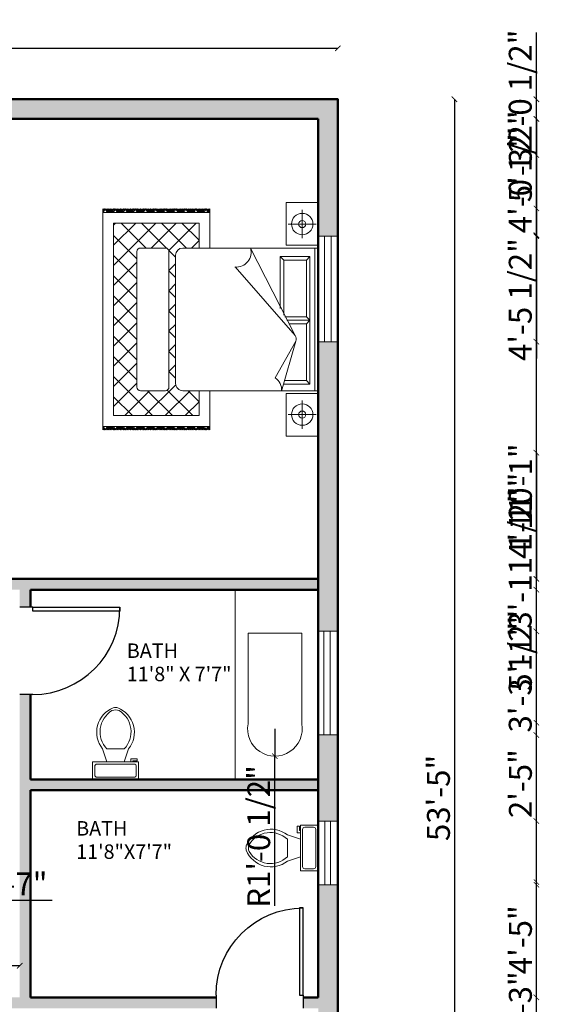
# Model space of a CAD drawing. Units: inches. Extents: x 1549 to 2410, y 1378 to 2139.
# Tile 6 of 6: x 2164 to 2410, y 1654 to 2106. Entities that reach past the tile are written whole.
import ezdxf

# ---------------------------------------------------------------- set-up
doc = ezdxf.new("R2010")
doc.units = ezdxf.units.IN
for name, color, linetype, lineweight in [('A-ANNO-DIMS', 2, 'Continuous', 18), ('A-AREA-IDEN', 7, 'Continuous', 18), ('A-DOOR', 4, 'Continuous', 25), ('A-FLOR-FIXT', 9, 'Continuous', 18), ('A-FURN', 8, 'Continuous', 18), ('A-WALL', 7, 'Continuous', 50), ('WINDOW', 2, 'Continuous', 18)]:
    doc.layers.add(name, color=color, linetype=linetype, lineweight=lineweight)
doc.layers.add('A-WALL-PATT', color=18, linetype='Continuous', lineweight=13, true_color=0x000000)
doc.styles.get("Standard").update_dxf_attribs({"font": 'arial.ttf'})
doc.dimstyles.new('ISO-25', dxfattribs={"dimtxt": 10.5, "dimasz": 2.5, "dimexe": 1.25, "dimexo": 0.625, "dimtad": 1, "dimdec": 0, "dimlunit": 4, "dimtxsty": 'Standard', "dimblk": 'ARCHTICK', "dimcen": 2.5, "dimse1": 1, "dimse2": 1, "dimclrd": 1, "dimclrt": 3, "dimadec": 0, "dimazin": 0, "dimtfac": 1, "dimtdec": 0, "dimtmove": 0, "dimatfit": 3, "dimfxl": 1, "dimarcsym": 0})

# ---------------------------------------------------------------- blocks, each defined once
blk = doc.blocks.new('*U5')
for p, q in [((9.5, -6), (9.5, -2)), ((-10, -8.5), (-8, -8.5)), ((-10, -9.5), (-10, -8.5)), ((-8, -8.5), (-8, -8)), ((-7, -8), (-7, -9.5)), ((-4, -8), (-6, -14)), ((4, -8), (6, -14)), ((-7, -9.5), (-10, -9.5)), ((4, -14), (-4, -14))]:
    blk.add_line(p, q)
blk.add_lwpolyline([(10.5, -8), (10.5, 0), (-10.5, 0), (-10.5, -8)], close=True)
for points in [[(-9.5, -2), (-9.5, -6)], [(8.5, -1), (-8.5, -1)], [(-8.5, -7), (8.5, -7)]]:
    blk.add_lwpolyline(points)
for centre, radius, start, end in [((-8.62, -1.88), 0.884, 81.8699, 188.1301), ((8.62, -1.88), 0.884, 351.8699, 98.1301), ((-8.62, -6.12), 0.884, 171.8699, 278.1301), ((8.62, -6.12), 0.884, 261.8699, 8.1301), ((3.52, -21.58), 12.17, 141.4691, 247.9714), ((4.2, -21.82), 11.33, 136.3677, 238.9468), ((-3.52, -21.58), 12.17, 292.0284, 38.5307), ((-4.2, -21.82), 11.33, 301.053, 43.6321), ((0, -27.88), 4, 245.7318, 294.2682), ((0, -29), 4, 254.8605, 285.1395)]:
    blk.add_arc(centre, radius, start, end)
blk = doc.blocks.new('*U3')
for p, q in [((0, 0), (0, -6)), ((40, 0), (40, -6))]:
    blk.add_line(p, q)
blk.add_lwpolyline([(0, 0), (0, 40), (1.75, 40), (1.75, 0)], close=True)
blk.add_arc((0, 0), 40, 0, 90)
blk = doc.blocks.new('A$C4CB008C5')
for p, q in [((0, 3.019), (0.6, 3.019)), ((0, 2.569), (0, 3.019)), ((0.304, 2.6), (0.304, 2.992)), ((0.6, 3.019), (0.6, 2.569)), ((0.64, 1.121), (0.64, 3.021)), ((0.64, 3.021), (2.64, 3.021)), ((0.64, 2.971), (2.64, 2.971)), ((0.759, 2.905), (2.547, 2.905)), ((0.759, 2.489), (0.759, 2.905)), ((0.759, 2.905), (0.809, 2.855)), ((1.603, 2.855), (1.653, 2.905)), ((1.653, 2.905), (1.653, 2.579)), ((1.653, 2.905), (1.703, 2.855)), ((2.497, 2.855), (2.547, 2.905)), ((2.547, 2.905), (2.547, 2.54)), ((2.64, 3.021), (2.64, 1.121)), ((3.279, 3.019), (2.679, 3.019)), ((2.679, 3.019), (2.679, 2.569)), ((2.975, 2.6), (2.975, 2.992)), ((3.279, 2.569), (3.279, 3.019)), ((0.106, 2.796), (0.503, 2.796)), ((0.809, 2.855), (1.603, 2.855)), ((0.809, 2.539), (0.809, 2.855)), ((1.603, 2.855), (1.603, 2.551)), ((1.703, 2.855), (1.703, 2.607)), ((1.703, 2.855), (2.497, 2.855)), ((2.497, 2.855), (2.497, 2.556)), ((3.174, 2.796), (2.776, 2.796)), ((0.64, 2.071), (1.866, 2.698)), ((0.906, 1.854), (1.866, 2.698)), ((1.946, 2.705), (2.646, 2.507)), ((1.946, 2.705), (2.46, 2.418)), ((0.6, 2.569), (0, 2.569)), ((0.809, 2.539), (0.759, 2.489)), ((1.49, 2.489), (0.759, 2.489)), ((1.58, 2.539), (0.809, 2.539)), ((2.679, 2.569), (3.279, 2.569)), ((0.907, 1.867), (0.919, 1.867)), ((0.09, 1.5), (0.64, 1.5)), ((0.09, 1.491), (0.099, 1.5)), ((0.09, 1.473), (0.116, 1.5)), ((0.09, 1.456), (0.134, 1.5)), ((0.09, 1.474), (0.09, 1.475)), ((0.09, 1.438), (0.126, 1.474)), ((0.117, 1.43), (0.09, 1.457)), ((0.14, 1.389), (0.09, 1.439)), ((0.09, 1.42), (0.099, 1.43)), ((0.14, 1.372), (0.09, 1.422)), ((0.09, 1.368), (0.14, 1.417)), ((0.14, 1.354), (0.09, 1.404)), ((0.09, 1.35), (0.14, 1.4)), ((0.14, 1.336), (0.09, 1.386)), ((0.09, 1.332), (0.14, 1.382)), ((0.14, 1.46), (0.108, 1.492)), ((0.117, 1.412), (0.14, 1.435)), ((0.14, 1.478), (0.118, 1.5)), ((0.14, 1.496), (0.135, 1.5)), ((0.14, 1.442), (0.135, 1.448)), ((0.14, 0), (0.14, 1.5)), ((2.64, 1.5), (3.19, 1.5)), ((3.14, 1.496), (3.144, 1.5)), ((3.14, 1.478), (3.162, 1.5)), ((3.14, 1.5), (3.14, 0)), ((3.14, 1.46), (3.171, 1.492)), ((3.14, 1.442), (3.145, 1.448)), ((3.14, 1.389), (3.19, 1.439)), ((3.162, 1.412), (3.14, 1.435)), ((3.14, 1.372), (3.19, 1.422)), ((3.189, 1.368), (3.14, 1.417)), ((3.14, 1.354), (3.19, 1.404)), ((3.19, 1.35), (3.14, 1.4)), ((3.14, 1.336), (3.19, 1.386)), ((3.19, 1.332), (3.14, 1.382)), ((3.19, 1.456), (3.145, 1.5)), ((3.19, 1.438), (3.154, 1.474)), ((3.162, 1.43), (3.19, 1.457)), ((3.19, 1.473), (3.163, 1.5)), ((3.19, 1.42), (3.18, 1.43)), ((3.19, 1.491), (3.181, 1.5)), ((3.189, 1.474), (3.19, 1.475)), ((0.09, 1.314), (0.14, 1.364)), ((0.09, 1.297), (0.126, 1.333)), ((0.09, 1.333), (0.09, 1.333)), ((0.117, 1.288), (0.09, 1.316)), ((0.14, 1.248), (0.09, 1.298)), ((0.09, 1.279), (0.099, 1.288)), ((0.14, 1.23), (0.09, 1.28)), ((0.09, 1.227), (0.14, 1.276)), ((0.14, 1.213), (0.09, 1.263)), ((0.09, 1.208), (0.14, 1.258)), ((0.14, 1.195), (0.09, 1.245)), ((0.14, 1.319), (0.108, 1.35)), ((0.117, 1.271), (0.14, 1.294)), ((0.14, 1.301), (0.135, 1.306)), ((0.29, 1.108), (0.532, 1.35)), ((0.29, 0.15), (0.29, 1.35)), ((0.29, 1.35), (0.64, 1.35)), ((0.674, 0.926), (0.29, 1.31)), ((0.64, 1.243), (0.533, 1.35)), ((2.632, 0.904), (2.99, 1.262)), ((2.64, 1.195), (2.795, 1.35)), ((2.64, 1.35), (2.99, 1.35)), ((2.99, 1.156), (2.795, 1.35)), ((2.99, 1.35), (2.99, 0.15)), ((3.19, 1.314), (3.14, 1.364)), ((3.14, 1.319), (3.171, 1.35)), ((3.14, 1.301), (3.145, 1.306)), ((3.14, 1.248), (3.19, 1.298)), ((3.162, 1.271), (3.14, 1.294)), ((3.14, 1.23), (3.19, 1.28)), ((3.189, 1.227), (3.14, 1.276)), ((3.14, 1.213), (3.19, 1.263)), ((3.19, 1.208), (3.14, 1.258)), ((3.14, 1.195), (3.19, 1.245)), ((3.19, 1.297), (3.154, 1.333)), ((3.162, 1.288), (3.19, 1.316)), ((3.19, 1.279), (3.18, 1.288)), ((3.189, 1.333), (3.19, 1.333)), ((0.09, 1.19), (0.14, 1.24)), ((0.09, 1.173), (0.14, 1.223)), ((0.09, 1.191), (0.09, 1.192)), ((0.09, 1.155), (0.126, 1.191)), ((0.117, 1.147), (0.09, 1.174)), ((0.14, 1.107), (0.09, 1.157)), ((0.09, 1.137), (0.099, 1.147)), ((0.14, 1.089), (0.09, 1.139)), ((0.09, 1.085), (0.14, 1.134)), ((0.14, 1.071), (0.09, 1.121)), ((0.09, 1.067), (0.14, 1.117)), ((0.14, 1.177), (0.108, 1.209)), ((0.117, 1.129), (0.14, 1.152)), ((0.14, 1.16), (0.135, 1.165)), ((0.29, 0.825), (0.64, 1.175)), ((2.99, 0.873), (2.64, 1.223)), ((3.19, 1.19), (3.14, 1.24)), ((3.19, 1.173), (3.14, 1.223)), ((3.14, 1.177), (3.171, 1.209)), ((3.14, 1.16), (3.145, 1.165)), ((3.14, 1.107), (3.19, 1.157)), ((3.162, 1.129), (3.14, 1.152)), ((3.14, 1.089), (3.19, 1.139)), ((3.189, 1.085), (3.14, 1.134)), ((3.14, 1.071), (3.19, 1.121)), ((3.19, 1.067), (3.14, 1.117)), ((3.19, 1.155), (3.154, 1.191)), ((3.162, 1.147), (3.19, 1.174)), ((3.19, 1.137), (3.18, 1.147)), ((3.189, 1.191), (3.19, 1.192)), ((0.14, 1.054), (0.09, 1.104)), ((0.09, 1.049), (0.14, 1.099)), ((0.09, 1.031), (0.14, 1.081)), ((0.09, 1.05), (0.09, 1.051)), ((0.09, 1.014), (0.126, 1.05)), ((0.117, 1.006), (0.09, 1.033)), ((0.14, 0.965), (0.09, 1.015)), ((0.09, 0.996), (0.099, 1.006)), ((0.14, 0.948), (0.09, 0.998)), ((0.09, 0.944), (0.14, 0.993)), ((0.14, 0.93), (0.09, 0.98)), ((0.09, 0.925), (0.14, 0.975)), ((0.14, 1.036), (0.108, 1.067)), ((0.117, 0.988), (0.14, 1.011)), ((0.14, 1.018), (0.135, 1.023)), ((0.64, 0.677), (0.29, 1.027)), ((0.673, 0.925), (0.769, 1.021)), ((2.54, 1.021), (0.74, 1.021)), ((0.955, 0.928), (0.861, 1.021)), ((0.959, 0.928), (1.052, 1.021)), ((1.238, 0.928), (1.144, 1.021)), ((1.241, 0.928), (1.335, 1.021)), ((1.52, 0.928), (1.427, 1.021)), ((1.524, 0.928), (1.618, 1.021)), ((1.803, 0.928), (1.71, 1.021)), ((1.807, 0.928), (1.9, 1.021)), ((2.086, 0.928), (1.993, 1.021)), ((2.09, 0.928), (2.183, 1.021)), ((2.369, 0.928), (2.276, 1.021)), ((2.373, 0.928), (2.466, 1.021)), ((2.99, 0.59), (2.557, 1.023)), ((2.64, 0.629), (2.99, 0.979)), ((3.14, 1.054), (3.19, 1.104)), ((3.19, 1.049), (3.14, 1.099)), ((3.19, 1.031), (3.14, 1.081)), ((3.14, 1.036), (3.171, 1.067)), ((3.14, 1.018), (3.145, 1.023)), ((3.14, 0.965), (3.19, 1.015)), ((3.162, 0.988), (3.14, 1.011)), ((3.14, 0.948), (3.19, 0.998)), ((3.189, 0.944), (3.14, 0.993)), ((3.14, 0.93), (3.19, 0.98)), ((3.19, 0.925), (3.14, 0.975)), ((3.19, 1.014), (3.154, 1.05)), ((3.162, 1.006), (3.19, 1.033)), ((3.19, 0.996), (3.18, 1.006)), ((3.189, 1.05), (3.19, 1.051)), ((0.14, 0.912), (0.09, 0.962)), ((0.09, 0.908), (0.14, 0.958)), ((0.09, 0.89), (0.14, 0.94)), ((0.09, 0.908), (0.09, 0.909)), ((0.09, 0.872), (0.126, 0.908)), ((0.117, 0.864), (0.09, 0.891)), ((0.14, 0.824), (0.09, 0.874)), ((0.09, 0.855), (0.099, 0.864)), ((0.14, 0.806), (0.09, 0.856)), ((0.09, 0.802), (0.14, 0.852)), ((0.14, 0.788), (0.09, 0.838)), ((0.09, 0.784), (0.14, 0.834)), ((0.14, 0.894), (0.108, 0.926)), ((0.117, 0.847), (0.14, 0.869)), ((0.14, 0.877), (0.135, 0.882)), ((0.29, 0.542), (0.643, 0.895)), ((0.64, 0.878), (0.64, 0.528)), ((0.69, 0.928), (2.59, 0.928)), ((2.64, 0.878), (2.64, 0.528)), ((3.14, 0.912), (3.19, 0.962)), ((3.19, 0.908), (3.14, 0.958)), ((3.19, 0.89), (3.14, 0.94)), ((3.14, 0.894), (3.171, 0.926)), ((3.14, 0.877), (3.145, 0.882)), ((3.14, 0.824), (3.19, 0.874)), ((3.162, 0.847), (3.14, 0.869)), ((3.14, 0.806), (3.19, 0.856)), ((3.189, 0.802), (3.14, 0.852)), ((3.14, 0.788), (3.19, 0.838)), ((3.19, 0.784), (3.14, 0.834)), ((3.19, 0.872), (3.154, 0.908)), ((3.162, 0.864), (3.19, 0.891)), ((3.19, 0.855), (3.18, 0.864)), ((3.189, 0.908), (3.19, 0.909)), ((0.14, 0.771), (0.09, 0.821)), ((0.09, 0.766), (0.14, 0.816)), ((0.09, 0.749), (0.14, 0.799)), ((0.09, 0.767), (0.09, 0.768)), ((0.09, 0.731), (0.126, 0.767)), ((0.117, 0.723), (0.09, 0.75)), ((0.14, 0.682), (0.09, 0.732)), ((0.09, 0.713), (0.099, 0.723)), ((0.14, 0.665), (0.09, 0.715)), ((0.09, 0.661), (0.14, 0.71)), ((0.14, 0.647), (0.09, 0.697)), ((0.09, 0.642), (0.14, 0.692)), ((0.14, 0.753), (0.108, 0.785)), ((0.117, 0.705), (0.14, 0.728)), ((0.14, 0.735), (0.135, 0.74)), ((0.884, 0.15), (0.29, 0.744)), ((2.443, 0.15), (2.99, 0.696)), ((3.14, 0.771), (3.19, 0.821)), ((3.19, 0.766), (3.14, 0.816)), ((3.19, 0.749), (3.14, 0.799)), ((3.14, 0.753), (3.171, 0.785)), ((3.14, 0.735), (3.145, 0.74)), ((3.14, 0.682), (3.19, 0.732)), ((3.162, 0.705), (3.14, 0.728)), ((3.14, 0.665), (3.19, 0.715)), ((3.189, 0.661), (3.14, 0.71)), ((3.14, 0.647), (3.19, 0.697)), ((3.19, 0.642), (3.14, 0.692)), ((3.19, 0.731), (3.154, 0.767)), ((3.162, 0.723), (3.19, 0.75)), ((3.19, 0.713), (3.18, 0.723)), ((3.189, 0.767), (3.19, 0.768)), ((0.14, 0.629), (0.09, 0.679)), ((0.09, 0.625), (0.14, 0.675)), ((0.09, 0.607), (0.14, 0.657)), ((0.09, 0.589), (0.126, 0.626)), ((0.09, 0.626), (0.09, 0.626)), ((0.117, 0.581), (0.09, 0.609)), ((0.14, 0.541), (0.09, 0.591)), ((0.09, 0.572), (0.099, 0.581)), ((0.14, 0.523), (0.09, 0.573)), ((0.09, 0.519), (0.14, 0.569)), ((0.14, 0.506), (0.09, 0.556)), ((0.14, 0.612), (0.108, 0.643)), ((0.117, 0.564), (0.14, 0.586)), ((0.14, 0.594), (0.135, 0.599)), ((0.29, 0.259), (0.64, 0.609)), ((2.99, 0.307), (2.64, 0.657)), ((3.14, 0.629), (3.19, 0.679)), ((3.19, 0.625), (3.14, 0.675)), ((3.19, 0.607), (3.14, 0.657)), ((3.14, 0.612), (3.171, 0.643)), ((3.14, 0.594), (3.145, 0.599)), ((3.14, 0.541), (3.19, 0.591)), ((3.162, 0.564), (3.14, 0.586)), ((3.14, 0.523), (3.19, 0.573)), ((3.189, 0.519), (3.14, 0.569)), ((3.14, 0.506), (3.19, 0.556)), ((3.19, 0.589), (3.154, 0.626)), ((3.162, 0.581), (3.19, 0.609)), ((3.19, 0.572), (3.18, 0.581)), ((3.189, 0.626), (3.19, 0.626)), ((0.09, 0.501), (0.14, 0.551)), ((0.14, 0.488), (0.09, 0.538)), ((0.09, 0.483), (0.14, 0.533)), ((0.09, 0.466), (0.14, 0.516)), ((0.09, 0.484), (0.09, 0.485)), ((0.09, 0.448), (0.126, 0.484)), ((0.117, 0.44), (0.09, 0.467)), ((0.14, 0.399), (0.09, 0.449)), ((0.09, 0.43), (0.099, 0.44)), ((0.14, 0.382), (0.09, 0.432)), ((0.09, 0.378), (0.14, 0.427)), ((0.14, 0.364), (0.09, 0.414)), ((0.14, 0.47), (0.108, 0.502)), ((0.117, 0.422), (0.14, 0.445)), ((0.14, 0.453), (0.135, 0.458)), ((0.601, 0.15), (0.29, 0.462)), ((0.463, 0.15), (0.791, 0.478)), ((0.69, 0.478), (2.59, 0.478)), ((0.746, 0.15), (1.074, 0.478)), ((1.167, 0.15), (0.839, 0.478)), ((1.029, 0.15), (1.357, 0.478)), ((1.45, 0.15), (1.122, 0.478)), ((1.312, 0.15), (1.64, 0.478)), ((1.733, 0.15), (1.405, 0.478)), ((1.595, 0.15), (1.923, 0.478)), ((2.016, 0.15), (1.688, 0.478)), ((1.878, 0.15), (2.206, 0.478)), ((2.298, 0.15), (1.97, 0.478)), ((2.16, 0.15), (2.488, 0.478)), ((2.581, 0.15), (2.253, 0.478)), ((2.864, 0.15), (2.536, 0.478)), ((3.19, 0.501), (3.14, 0.551)), ((3.14, 0.488), (3.19, 0.538)), ((3.19, 0.483), (3.14, 0.533)), ((3.19, 0.466), (3.14, 0.516)), ((3.14, 0.47), (3.171, 0.502)), ((3.14, 0.453), (3.145, 0.458)), ((3.14, 0.399), (3.19, 0.449)), ((3.162, 0.422), (3.14, 0.445)), ((3.14, 0.382), (3.19, 0.432)), ((3.189, 0.378), (3.14, 0.427)), ((3.14, 0.364), (3.19, 0.414)), ((3.19, 0.448), (3.154, 0.484)), ((3.162, 0.44), (3.19, 0.467)), ((3.19, 0.43), (3.18, 0.44)), ((3.189, 0.484), (3.19, 0.485)), ((0.09, 0.36), (0.14, 0.41)), ((0.14, 0.346), (0.09, 0.396)), ((0.09, 0.342), (0.14, 0.392)), ((0.09, 0.324), (0.14, 0.374)), ((0.09, 0.307), (0.126, 0.343)), ((0.09, 0.343), (0.09, 0.343)), ((0.117, 0.299), (0.09, 0.326)), ((0.14, 0.258), (0.09, 0.308)), ((0.09, 0.289), (0.099, 0.299)), ((0.14, 0.24), (0.09, 0.29)), ((0.09, 0.237), (0.14, 0.286)), ((0.14, 0.329), (0.108, 0.36)), ((0.117, 0.281), (0.14, 0.304)), ((0.14, 0.311), (0.135, 0.316)), ((2.726, 0.15), (2.99, 0.414)), ((3.19, 0.36), (3.14, 0.41)), ((3.14, 0.346), (3.19, 0.396)), ((3.19, 0.342), (3.14, 0.392)), ((3.19, 0.324), (3.14, 0.374)), ((3.14, 0.329), (3.171, 0.36)), ((3.14, 0.311), (3.145, 0.316)), ((3.14, 0.258), (3.19, 0.308)), ((3.162, 0.281), (3.14, 0.304)), ((3.14, 0.24), (3.19, 0.29)), ((3.189, 0.237), (3.14, 0.286)), ((3.19, 0.307), (3.154, 0.343)), ((3.162, 0.299), (3.19, 0.326)), ((3.19, 0.289), (3.18, 0.299)), ((3.189, 0.343), (3.19, 0.343)), ((0.14, 0.223), (0.09, 0.273)), ((0.09, 0.218), (0.14, 0.268)), ((0.14, 0.205), (0.09, 0.255)), ((0.09, 0.201), (0.14, 0.251)), ((0.09, 0.183), (0.14, 0.233)), ((0.09, 0.201), (0.09, 0.202)), ((0.09, 0.165), (0.126, 0.201)), ((0.117, 0.157), (0.09, 0.184)), ((0.14, 0.117), (0.09, 0.167)), ((0.09, 0.148), (0.099, 0.157)), ((0.14, 0.099), (0.09, 0.149)), ((0.09, 0.095), (0.14, 0.144)), ((0.14, 0.187), (0.108, 0.219)), ((0.117, 0.139), (0.14, 0.162)), ((0.14, 0.17), (0.135, 0.175)), ((0.318, 0.15), (0.29, 0.179)), ((2.99, 0.15), (0.29, 0.15)), ((3.14, 0.223), (3.19, 0.273)), ((3.19, 0.218), (3.14, 0.268)), ((3.14, 0.205), (3.19, 0.255)), ((3.19, 0.201), (3.14, 0.251)), ((3.19, 0.183), (3.14, 0.233)), ((3.14, 0.187), (3.171, 0.219)), ((3.14, 0.17), (3.145, 0.175)), ((3.14, 0.117), (3.19, 0.167)), ((3.162, 0.139), (3.14, 0.162)), ((3.14, 0.099), (3.19, 0.149)), ((3.189, 0.095), (3.14, 0.144)), ((3.19, 0.165), (3.154, 0.201)), ((3.162, 0.157), (3.19, 0.184)), ((3.19, 0.148), (3.18, 0.157)), ((3.189, 0.201), (3.19, 0.202)), ((0.14, 0.081), (0.09, 0.131)), ((0.09, 0.077), (0.14, 0.127)), ((0.14, 0.064), (0.09, 0.114)), ((0.09, 0.059), (0.14, 0.109)), ((0.09, 0.041), (0.14, 0.091)), ((0.09, 0.06), (0.09, 0.061)), ((0.09, 0.024), (0.126, 0.06)), ((0.117, 0.016), (0.09, 0.043)), ((0.115, 0), (0.09, 0.025)), ((0.09, 0.006), (0.099, 0.016)), ((0.097, 0), (0.09, 0.008)), ((0.14, 0.046), (0.108, 0.078)), ((0.119, 0), (0.14, 0.021)), ((0.14, 0.028), (0.135, 0.033)), ((0.137, 0), (0.14, 0.003)), ((3.14, 0.081), (3.19, 0.131)), ((3.19, 0.077), (3.14, 0.127)), ((3.14, 0.064), (3.19, 0.114)), ((3.19, 0.059), (3.14, 0.109)), ((3.19, 0.041), (3.14, 0.091)), ((3.14, 0.046), (3.171, 0.078)), ((3.14, 0.028), (3.145, 0.033)), ((3.16, 0), (3.14, 0.021)), ((3.143, 0), (3.14, 0.003)), ((3.19, 0.024), (3.154, 0.06)), ((3.162, 0.016), (3.19, 0.043)), ((3.164, 0), (3.19, 0.025)), ((3.19, 0.006), (3.18, 0.016)), ((3.182, 0), (3.19, 0.008)), ((3.189, 0.06), (3.19, 0.061)), ((0.09, 0), (3.19, 0))]:
    blk.add_line(p, q)
for centre, radius in [((0.304, 2.796), 0.15), ((2.975, 2.796), 0.15), ((0.304, 2.796), 0.05), ((2.975, 2.796), 0.05)]:
    blk.add_circle(centre, radius)
for centre, radius, start, end in [((1.915, 2.61), 0.1, 71.7215, 119.0799), ((2.626, 2.31), 0.198, 84.1725, 146.9889), ((0.7, 1.873), 0.207, 354.6422, 106.9775), ((0.74, 1.121), 0.1, 180, 270), ((2.54, 1.121), 0.1, 270, 0), ((0.69, 0.878), 0.05, 90, 180), ((2.59, 0.878), 0.05, 0, 90), ((0.69, 0.528), 0.05, 180, 270), ((2.59, 0.528), 0.05, 270, 0)]:
    blk.add_arc(centre, radius, start, end)
blk = doc.blocks.new('_ArchTick')
at = {"color": 0, "linetype": 'ByBlock', "const_width": 0.15}
blk.add_lwpolyline([(-0.5, -0.5), (0.5, 0.5)], dxfattribs=at)
blk = doc.blocks.new('*D13')
at = {"layer": 'A-ANNO-DIMS', "color": 0, "lineweight": -2, "transparency": 16777216}
blk.add_line((1688.62, 2092.38), (2309.62, 2092.38), dxfattribs=at)
at = {"layer": 'Defpoints', "color": 0, "transparency": 16777216}
for p in [(2309.62, 2092.38), (1688.62, 2069.01), (2309.62, 2069.01)]:
    blk.add_point(p, dxfattribs=at)
at = {"layer": 'A-ANNO-DIMS', "color": 0, "lineweight": -2, "transparency": 16777216, "xscale": 2.5, "yscale": 2.5, "zscale": 2.5, "rotation": 180}
blk.add_blockref('_ArchTick', (1688.62, 2092.38), dxfattribs=at)
at = {"layer": 'A-ANNO-DIMS', "color": 0, "lineweight": -2, "transparency": 16777216, "xscale": 2.5, "yscale": 2.5, "zscale": 2.5}
blk.add_blockref('_ArchTick', (2309.62, 2092.38), dxfattribs=at)
at = {"layer": 'A-ANNO-DIMS', "color": 0, "transparency": 16777216, "insert": (1999.12, 2098.36), "char_height": 10.5, "attachment_point": 5}
blk.add_mtext('51\'-9"', dxfattribs=at)
blk = doc.blocks.new('*D14')
at = {"layer": 'A-ANNO-DIMS', "color": 0, "lineweight": -2, "transparency": 16777216}
blk.add_line((2363.11, 2069.01), (2363.11, 1428.01), dxfattribs=at)
at = {"layer": 'Defpoints', "color": 0, "transparency": 16777216}
for p in [(2309.62, 2069.01), (2309.62, 1428.01), (2363.11, 1428.01)]:
    blk.add_point(p, dxfattribs=at)
at = {"layer": 'A-ANNO-DIMS', "color": 0, "lineweight": -2, "transparency": 16777216, "xscale": 2.5, "yscale": 2.5, "zscale": 2.5}
for p, rotation in [((2363.11, 2069.01), 90), ((2363.11, 1428.01), 270)]:
    blk.add_blockref('_ArchTick', p, dxfattribs=dict(at, rotation=rotation))
at = {"layer": 'A-ANNO-DIMS', "color": 0, "transparency": 16777216, "insert": (2357.12, 1748.51), "char_height": 10.5, "attachment_point": 5, "rotation": 90}
blk.add_mtext('53\'-5"', dxfattribs=at)
blk = doc.blocks.new('*D23')
at = {"layer": 'A-ANNO-DIMS', "color": 1, "lineweight": -2, "transparency": 16777216}
for p, q in [((1968.32, 1701.64), (2059.32, 1701.64)), ((2059.32, 1701.64), (2178.47, 1701.64))]:
    blk.add_line(p, q, dxfattribs=at)
at = {"layer": 'Defpoints', "color": 0, "transparency": 16777216}
for p in [(1968.32, 1715.29), (2059.32, 1715.29), (2059.32, 1701.64)]:
    blk.add_point(p, dxfattribs=at)
at = {"layer": 'A-ANNO-DIMS', "color": 1, "lineweight": -2, "transparency": 16777216, "xscale": 2.5, "yscale": 2.5, "zscale": 2.5, "rotation": 180}
blk.add_blockref('_ArchTick', (1968.32, 1701.64), dxfattribs=at)
at = {"layer": 'A-ANNO-DIMS', "color": 1, "lineweight": -2, "transparency": 16777216, "xscale": 2.5, "yscale": 2.5, "zscale": 2.5}
blk.add_blockref('_ArchTick', (2059.32, 1701.64), dxfattribs=at)
at = {"layer": 'A-ANNO-DIMS', "color": 3, "transparency": 16777216, "insert": (2120.15, 1707.7), "char_height": 10.5, "attachment_point": 5}
blk.add_mtext('DINING SET 7\'-7"', dxfattribs=at)
blk = doc.blocks.new('*D26')
at = {"layer": 'A-ANNO-DIMS', "color": 1, "lineweight": -2, "transparency": 16777216}
blk.add_line((2163.62, 1671.5), (2097.13, 1671.5), dxfattribs=at)
at = {"layer": 'Defpoints', "color": 0, "transparency": 16777216}
for p in [(2097.13, 1684.51), (2163.62, 1684.51), (2097.13, 1671.5)]:
    blk.add_point(p, dxfattribs=at)
at = {"layer": 'A-ANNO-DIMS', "color": 1, "lineweight": -2, "transparency": 16777216, "xscale": 2.5, "yscale": 2.5, "zscale": 2.5, "rotation": 180}
blk.add_blockref('_ArchTick', (2097.13, 1671.5), dxfattribs=at)
at = {"layer": 'A-ANNO-DIMS', "color": 1, "lineweight": -2, "transparency": 16777216, "xscale": 2.5, "yscale": 2.5, "zscale": 2.5}
blk.add_blockref('_ArchTick', (2163.62, 1671.5), dxfattribs=at)
at = {"layer": 'A-ANNO-DIMS', "color": 3, "transparency": 16777216, "insert": (2130.37, 1677.55), "char_height": 10.5, "attachment_point": 5}
blk.add_mtext('5\'-6 1/2"', dxfattribs=at)
blk = doc.blocks.new('*D41')
at = {"layer": 'A-ANNO-DIMS', "color": 1, "lineweight": -2, "transparency": 16777216}
blk.add_line((2400.7, 1597.64), (2400.7, 1708.66), dxfattribs=at)
at = {"layer": 'Defpoints', "color": 0, "transparency": 16777216}
for p in [(2309.62, 1708.66), (2400.7, 1708.66), (2309.62, 1597.64)]:
    blk.add_point(p, dxfattribs=at)
at = {"layer": 'A-ANNO-DIMS', "color": 1, "lineweight": -2, "transparency": 16777216, "xscale": 2.5, "yscale": 2.5, "zscale": 2.5}
for p, rotation in [((2400.7, 1708.66), 90), ((2400.7, 1597.64), 270)]:
    blk.add_blockref('_ArchTick', p, dxfattribs=dict(at, rotation=rotation))
at = {"layer": 'A-ANNO-DIMS', "color": 3, "transparency": 16777216, "insert": (2394.71, 1653.15), "char_height": 10.5, "attachment_point": 5, "rotation": 90}
blk.add_mtext('9\'-3"', dxfattribs=at)
blk = doc.blocks.new('*D42')
at = {"layer": 'A-ANNO-DIMS', "color": 1, "lineweight": -2, "transparency": 16777216}
for p, q in [((2400.7, 1737.9), (2400.7, 1769.74)), ((2400.7, 1708.66), (2400.7, 1737.9))]:
    blk.add_line(p, q, dxfattribs=at)
at = {"layer": 'Defpoints', "color": 0, "transparency": 16777216}
for p in [(2309.62, 1737.9), (2400.7, 1737.9), (2309.62, 1708.66)]:
    blk.add_point(p, dxfattribs=at)
at = {"layer": 'A-ANNO-DIMS', "color": 1, "lineweight": -2, "transparency": 16777216, "xscale": 2.5, "yscale": 2.5, "zscale": 2.5}
for p, rotation in [((2400.7, 1737.9), 90), ((2400.7, 1708.66), 270)]:
    blk.add_blockref('_ArchTick', p, dxfattribs=dict(at, rotation=rotation))
at = {"layer": 'A-ANNO-DIMS', "color": 3, "transparency": 16777216, "insert": (2394.72, 1755.07), "char_height": 10.5, "attachment_point": 5, "rotation": 90}
blk.add_mtext('2\'-5"', dxfattribs=at)
blk = doc.blocks.new('*D43')
at = {"layer": 'A-ANNO-DIMS', "color": 1, "lineweight": -2, "transparency": 16777216}
for p, q in [((2400.7, 1777.38), (2400.7, 1833.5)), ((2400.7, 1737.9), (2400.7, 1777.38))]:
    blk.add_line(p, q, dxfattribs=at)
at = {"layer": 'Defpoints', "color": 0, "transparency": 16777216}
for p in [(2309.62, 1777.38), (2400.7, 1777.38), (2309.62, 1737.9)]:
    blk.add_point(p, dxfattribs=at)
at = {"layer": 'A-ANNO-DIMS', "color": 1, "lineweight": -2, "transparency": 16777216, "xscale": 2.5, "yscale": 2.5, "zscale": 2.5}
for p, rotation in [((2400.7, 1777.38), 90), ((2400.7, 1737.9), 270)]:
    blk.add_blockref('_ArchTick', p, dxfattribs=dict(at, rotation=rotation))
at = {"layer": 'A-ANNO-DIMS', "color": 3, "transparency": 16777216, "insert": (2394.65, 1806.69), "char_height": 10.5, "attachment_point": 5, "rotation": 90}
blk.add_mtext('3\'-3 1/2"', dxfattribs=at)
blk = doc.blocks.new('*D44')
at = {"layer": 'A-ANNO-DIMS', "color": 1, "lineweight": -2, "transparency": 16777216}
for p, q in [((2400.7, 1824.93), (2400.7, 1889.2)), ((2400.7, 1777.38), (2400.7, 1824.93))]:
    blk.add_line(p, q, dxfattribs=at)
at = {"layer": 'Defpoints', "color": 0, "transparency": 16777216}
for p in [(2309.62, 1824.93), (2400.7, 1824.93), (2309.62, 1777.38)]:
    blk.add_point(p, dxfattribs=at)
at = {"layer": 'A-ANNO-DIMS', "color": 1, "lineweight": -2, "transparency": 16777216, "xscale": 2.5, "yscale": 2.5, "zscale": 2.5}
for p, rotation in [((2400.7, 1824.93), 90), ((2400.7, 1777.38), 270)]:
    blk.add_blockref('_ArchTick', p, dxfattribs=dict(at, rotation=rotation))
at = {"layer": 'A-ANNO-DIMS', "color": 3, "transparency": 16777216, "insert": (2394.65, 1858.32), "char_height": 10.5, "attachment_point": 5, "rotation": 90}
blk.add_mtext('3\'-11 1/2"', dxfattribs=at)
blk = doc.blocks.new('*D45')
at = {"layer": 'A-ANNO-DIMS', "color": 1, "lineweight": -2, "transparency": 16777216}
blk.add_line((2400.7, 1824.93), (2400.7, 1957.79), dxfattribs=at)
at = {"layer": 'Defpoints', "color": 0, "transparency": 16777216}
for p in [(2309.62, 1957.79), (2400.7, 1957.79), (2309.62, 1824.93)]:
    blk.add_point(p, dxfattribs=at)
at = {"layer": 'A-ANNO-DIMS', "color": 1, "lineweight": -2, "transparency": 16777216, "xscale": 2.5, "yscale": 2.5, "zscale": 2.5}
for p, rotation in [((2400.7, 1957.79), 90), ((2400.7, 1824.93), 270)]:
    blk.add_blockref('_ArchTick', p, dxfattribs=dict(at, rotation=rotation))
at = {"layer": 'A-ANNO-DIMS', "color": 3, "transparency": 16777216, "insert": (2394.81, 1891.36), "char_height": 10.5, "attachment_point": 5, "rotation": 90}
blk.add_mtext('11\'-1"', dxfattribs=at)
blk = doc.blocks.new('*D46')
at = {"layer": 'A-ANNO-DIMS', "color": 1, "lineweight": -2, "transparency": 16777216}
for p, q in [((2400.7, 2006.22), (2400.7, 2062.77)), ((2400.7, 1957.79), (2400.7, 2006.22))]:
    blk.add_line(p, q, dxfattribs=at)
at = {"layer": 'Defpoints', "color": 0, "transparency": 16777216}
for p in [(2309.62, 2006.22), (2400.7, 2006.22), (2309.62, 1957.79)]:
    blk.add_point(p, dxfattribs=at)
at = {"layer": 'A-ANNO-DIMS', "color": 1, "lineweight": -2, "transparency": 16777216, "xscale": 2.5, "yscale": 2.5, "zscale": 2.5}
for p, rotation in [((2400.7, 2006.22), 90), ((2400.7, 1957.79), 270)]:
    blk.add_blockref('_ArchTick', p, dxfattribs=dict(at, rotation=rotation))
at = {"layer": 'A-ANNO-DIMS', "color": 3, "transparency": 16777216, "insert": (2394.65, 2035.74), "char_height": 10.5, "attachment_point": 5, "rotation": 90}
blk.add_mtext('4\'-0 1/2"', dxfattribs=at)
blk = doc.blocks.new('*D47')
at = {"layer": 'A-ANNO-DIMS', "color": 1, "lineweight": -2, "transparency": 16777216}
blk.add_line((2400.7, 2006.22), (2400.7, 2069.01), dxfattribs=at)
at = {"layer": 'Defpoints', "color": 0, "transparency": 16777216}
for p in [(2309.62, 2069.01), (2400.7, 2069.01), (2309.62, 2006.22)]:
    blk.add_point(p, dxfattribs=at)
at = {"layer": 'A-ANNO-DIMS', "color": 1, "lineweight": -2, "transparency": 16777216, "xscale": 2.5, "yscale": 2.5, "zscale": 2.5}
for p, rotation in [((2400.7, 2069.01), 90), ((2400.7, 2006.22), 270)]:
    blk.add_blockref('_ArchTick', p, dxfattribs=dict(at, rotation=rotation))
at = {"layer": 'A-ANNO-DIMS', "color": 3, "transparency": 16777216, "insert": (2394.71, 2037.62), "char_height": 10.5, "attachment_point": 5, "rotation": 90}
blk.add_mtext('5\'-3"', dxfattribs=at)
blk = doc.blocks.new('*D48')
at = {"layer": 'A-ANNO-DIMS', "color": 1, "lineweight": -2, "transparency": 16777216}
for p, q in [((2400.7, 2060.01), (2400.7, 2006.66)), ((2400.7, 2006.66), (2400.7, 1950.11))]:
    blk.add_line(p, q, dxfattribs=at)
at = {"layer": 'Defpoints', "color": 0, "transparency": 16777216}
for p in [(1914.62, 2060.01), (1914.62, 2006.66), (2400.7, 2006.66)]:
    blk.add_point(p, dxfattribs=at)
at = {"layer": 'A-ANNO-DIMS', "color": 1, "lineweight": -2, "transparency": 16777216, "xscale": 2.5, "yscale": 2.5, "zscale": 2.5}
for p, rotation in [((2400.7, 2060.01), 90), ((2400.7, 2006.66), 270)]:
    blk.add_blockref('_ArchTick', p, dxfattribs=dict(at, rotation=rotation))
at = {"layer": 'A-ANNO-DIMS', "color": 3, "transparency": 16777216, "insert": (2394.65, 1977.14), "char_height": 10.5, "attachment_point": 5, "rotation": 90}
blk.add_mtext('4\'-5 1/2"', dxfattribs=at)
blk = doc.blocks.new('*D54')
at = {"layer": 'A-ANNO-DIMS', "color": 1, "lineweight": -2, "transparency": 16777216}
blk.add_line((2400.7, 1906.88), (2400.7, 1849.01), dxfattribs=at)
at = {"layer": 'Defpoints', "color": 0, "transparency": 16777216}
for p in [(2082.62, 1906.88), (2082.62, 1849.01), (2400.7, 1849.01)]:
    blk.add_point(p, dxfattribs=at)
at = {"layer": 'A-ANNO-DIMS', "color": 1, "lineweight": -2, "transparency": 16777216, "xscale": 2.5, "yscale": 2.5, "zscale": 2.5}
for p, rotation in [((2400.7, 1906.88), 90), ((2400.7, 1849.01), 270)]:
    blk.add_blockref('_ArchTick', p, dxfattribs=dict(at, rotation=rotation))
at = {"layer": 'A-ANNO-DIMS', "color": 3, "transparency": 16777216, "insert": (2394.72, 1877.94), "char_height": 10.5, "attachment_point": 5, "rotation": 90}
blk.add_mtext('4\'-10"', dxfattribs=at)
blk = doc.blocks.new('*D59')
at = {"layer": 'A-ANNO-DIMS', "color": 1, "lineweight": -2, "transparency": 16777216}
blk.add_line((2400.7, 1782.99), (2400.7, 1844.01), dxfattribs=at)
at = {"layer": 'Defpoints', "color": 0, "transparency": 16777216}
for p in [(1833.98, 1844.01), (2400.7, 1844.01), (1833.98, 1782.99)]:
    blk.add_point(p, dxfattribs=at)
at = {"layer": 'A-ANNO-DIMS', "color": 1, "lineweight": -2, "transparency": 16777216, "xscale": 2.5, "yscale": 2.5, "zscale": 2.5}
for p, rotation in [((2400.7, 1844.01), 90), ((2400.7, 1782.99), 270)]:
    blk.add_blockref('_ArchTick', p, dxfattribs=dict(at, rotation=rotation))
at = {"layer": 'A-ANNO-DIMS', "color": 3, "transparency": 16777216, "insert": (2394.72, 1813.5), "char_height": 10.5, "attachment_point": 5, "rotation": 90}
blk.add_mtext('5\'-1"', dxfattribs=at)
blk = doc.blocks.new('*D60')
at = {"layer": 'A-ANNO-DIMS', "color": 1, "lineweight": -2, "transparency": 16777216}
blk.add_line((2400.7, 1657.01), (2400.7, 1709.88), dxfattribs=at)
at = {"layer": 'Defpoints', "color": 0, "transparency": 16777216}
for p in [(1870.93, 1709.88), (2400.7, 1709.88), (1870.93, 1657.01)]:
    blk.add_point(p, dxfattribs=at)
at = {"layer": 'A-ANNO-DIMS', "color": 1, "lineweight": -2, "transparency": 16777216, "xscale": 2.5, "yscale": 2.5, "zscale": 2.5}
for p, rotation in [((2400.7, 1709.88), 90), ((2400.7, 1657.01), 270)]:
    blk.add_blockref('_ArchTick', p, dxfattribs=dict(at, rotation=rotation))
at = {"layer": 'A-ANNO-DIMS', "color": 3, "transparency": 16777216, "insert": (2394.74, 1683.45), "char_height": 10.5, "attachment_point": 5, "rotation": 90}
blk.add_mtext('4\'-5"', dxfattribs=at)
blk = doc.blocks.new('*D66')
at = {"layer": 'A-ANNO-DIMS', "color": 1, "lineweight": -2, "transparency": 16777216}
for p, q in [((2400.7, 2043.41), (2400.7, 2099.71)), ((2400.7, 2018.94), (2400.7, 2043.41))]:
    blk.add_line(p, q, dxfattribs=at)
at = {"layer": 'Defpoints', "color": 0, "transparency": 16777216}
for p in [(2087.62, 2043.41), (2400.7, 2043.41), (2087.62, 2018.94)]:
    blk.add_point(p, dxfattribs=at)
at = {"layer": 'A-ANNO-DIMS', "color": 1, "lineweight": -2, "transparency": 16777216, "xscale": 2.5, "yscale": 2.5, "zscale": 2.5}
for p, rotation in [((2400.7, 2043.41), 90), ((2400.7, 2018.94), 270)]:
    blk.add_blockref('_ArchTick', p, dxfattribs=dict(at, rotation=rotation))
at = {"layer": 'A-ANNO-DIMS', "color": 3, "transparency": 16777216, "insert": (2394.65, 2072.81), "char_height": 10.5, "attachment_point": 5, "rotation": 90}
blk.add_mtext('2\'-0 1/2"', dxfattribs=at)
blk = doc.blocks.new('*D67')
at = {"layer": 'A-ANNO-DIMS', "color": 1, "lineweight": -2, "transparency": 16777216}
for p in [(2280.71, 1780.19), (2280.71, 1698.99)]:
    blk.add_line(p, (2280.71, 1767.67), dxfattribs=at)
at = {"layer": 'Defpoints', "color": 0, "transparency": 16777216}
for p in [(2280.71, 1780.19), (2280.71, 1767.67)]:
    blk.add_point(p, dxfattribs=at)
at = {"layer": 'A-ANNO-DIMS', "color": 1, "lineweight": -2, "transparency": 16777216, "xscale": 2.5, "yscale": 2.5, "zscale": 2.5, "rotation": 90}
blk.add_blockref('_ArchTick', (2280.71, 1767.67), dxfattribs=at)
at = {"layer": 'A-ANNO-DIMS', "color": 3, "transparency": 16777216, "insert": (2274.65, 1730.83), "char_height": 10.5, "attachment_point": 5, "rotation": 90}
blk.add_mtext('R1\'-0 1/2"', dxfattribs=at)

msp = doc.modelspace()

# ---------------------------------------------------------------- hatches: boundary and pattern name
at = {"layer": 'A-WALL-PATT'}
h = msp.add_hatch(color=256, dxfattribs=at)
h.dxf.hatch_style = 1
h.paths.add_polyline_path([(1760, 2069.01), (1688.62, 2069.01), (1688.62, 2003.68), (1697.62, 2003.68), (1697.62, 2060.01), (1760, 2060.01)])
h.paths.add_polyline_path([(2309.62, 2069.01), (1807.68, 2069.01), (1807.68, 2060.01), (1909.62, 2060.01), (1909.62, 2040.27), (1914.62, 2040.27), (1914.62, 2060.01), (2082.62, 2060.01), (2082.62, 2043.41), (2087.62, 2043.41), (2087.62, 2060.01), (2300.62, 2060.01), (2300.62, 2006.22), (2309.62, 2006.22)])
h.paths.add_polyline_path([(1914.62, 1607.36), (1909.62, 1607.36), (1909.62, 1437.01), (1914.62, 1437.01)])
h.paths.add_polyline_path([(1697.62, 1536.06), (1688.62, 1536.06), (1688.62, 1428.01), (1745.28, 1428.01), (1745.28, 1437.01), (1697.62, 1437.01)])
h.paths.add_polyline_path([(2130.61, 1437.01), (2082.62, 1437.01), (2082.62, 1428.01), (2130.61, 1428.01)])
h.paths.add_polyline_path([(2309.62, 1544.51), (2302.25, 1544.51), (2302.25, 1524.81), (2300.62, 1524.81), (2300.62, 1523.51), (2302.17, 1523.51), (2302.17, 1503.88), (2300.62, 1503.88), (2300.62, 1437.01), (2193.34, 1437.01), (2193.34, 1428.01), (2309.62, 1428.01)])
h.paths.add_polyline_path([(2309.62, 1708.66), (2300.62, 1708.66), (2300.62, 1657.01), (2293.7, 1657.01), (2293.7, 1652.01), (2300.62, 1652.01), (2300.62, 1611.18), (2302.17, 1611.18), (2302.17, 1597.64), (2309.62, 1597.64)])
h.paths.add_polyline_path([(2309.62, 1777.38), (2300.62, 1777.38), (2300.62, 1737.9), (2309.62, 1737.9)])
h.paths.add_polyline_path([(2300.62, 1757.01), (2168.62, 1757.01), (2168.62, 1795.96), (2163.62, 1795.96), (2163.62, 1657.01), (2082.62, 1657.01), (2082.62, 1641.99), (2087.62, 1641.99), (2087.62, 1652.01), (2253.7, 1652.01), (2253.7, 1657.01), (2168.62, 1657.01), (2168.62, 1752.01), (2300.62, 1752.01)])
h.paths.add_polyline_path([(2309.62, 1957.79), (2300.62, 1957.79), (2300.62, 1935.33), (2300.62, 1824.93), (2309.62, 1824.93)])
h.paths.add_polyline_path([(2300.62, 1849.01), (2137.17, 1849.01), (2137.17, 1844.01), (2163.62, 1844.01), (2163.62, 1835.96), (2168.62, 1835.96), (2168.62, 1844.01), (2300.62, 1844.01)])
h.paths.add_polyline_path([(2211.06, 1800.23), (2261.76, 1800.23), (2261.76, 1810.41), (2211.06, 1810.41)], flags=9)
h.paths.add_polyline_path([(2211.1, 1811.05), (2239.18, 1811.05), (2239.18, 1821.02), (2211.1, 1821.02)], flags=9)
h.paths.add_polyline_path([(2187.84, 1718.73), (2233.38, 1718.73), (2233.38, 1728.91), (2187.84, 1728.91)], flags=25)
h.paths.add_polyline_path([(2187.88, 1729.56), (2215.96, 1729.56), (2215.96, 1739.52), (2187.88, 1739.52)], flags=25)
h.paths.add_polyline_path([(1720.01, 1609.74), (1775.87, 1609.74), (1775.87, 1619.93), (1720.01, 1619.93)], flags=9)
h.paths.add_polyline_path([(1719.99, 1620.4), (1782.23, 1620.4), (1782.23, 1630.72), (1719.99, 1630.72)], flags=9)
h.paths.add_polyline_path([(2092.97, 1541.04), (2148.83, 1541.04), (2148.83, 1551.23), (2092.97, 1551.23)], flags=9)
h.paths.add_polyline_path([(2092.94, 1551.69), (2155.19, 1551.69), (2155.19, 1562.02), (2092.94, 1562.02)], flags=9)
h.paths.add_polyline_path([(1759.73, 1747.67), (1815.59, 1747.67), (1815.59, 1757.85), (1759.73, 1757.85)], flags=9)
h.paths.add_polyline_path([(1759.71, 1758.32), (1790.48, 1758.32), (1790.48, 1768.63), (1759.71, 1768.63)], flags=9)
h.paths.add_polyline_path([(1940.79, 1793.43), (1996.65, 1793.43), (1996.65, 1803.61), (1940.79, 1803.61)], flags=9)
h.paths.add_polyline_path([(1940.77, 1804.08), (2006.11, 1804.08), (2006.11, 1814.4), (1940.77, 1814.4)], flags=9)
h.paths.add_polyline_path([(2094.62, 1963.23), (2150.43, 1963.23), (2150.43, 1973.25), (2094.62, 1973.25)], flags=9)
h.paths.add_polyline_path([(2094.57, 1973.75), (2156.81, 1973.75), (2156.81, 1984.07), (2094.57, 1984.07)], flags=9)
h.paths.add_polyline_path([(1943.36, 1930.19), (2000.28, 1930.19), (2000.28, 1940.37), (1943.36, 1940.37)], flags=9)
h.paths.add_polyline_path([(1943.34, 1940.85), (1987.53, 1940.85), (1987.53, 1951.15), (1943.34, 1951.15)], flags=9)
h.paths.add_polyline_path([(1803.94, 1971.5), (1857.22, 1971.5), (1857.22, 1981.68), (1803.94, 1981.68)], flags=9)
h.paths.add_polyline_path([(1803.92, 1982.16), (1866.16, 1982.16), (1866.16, 1992.47), (1803.92, 1992.47)], flags=9)

# ---------------------------------------------------------------- linework, layer by layer
at = {"layer": 'A-FLOR-FIXT'}
for p, q in [((2262.45, 1757.01), (2262.45, 1844.01)), ((2268.39, 1824.12), (2293.02, 1824.12)), ((2268.39, 1824.12), (2268.39, 1782.47)), ((2293.02, 1824.12), (2293.02, 1782.47))]:
    msp.add_line(p, q, dxfattribs=at)
msp.add_arc((2280.71, 1780.19), 12.53, 169.534, 10.466, dxfattribs=at)
at = {"layer": 'A-WALL'}
for p, q in [((2087.62, 2060.01), (2300.62, 2060.01)), ((2300.62, 2060.01), (2300.62, 1657.01)), ((2137.17, 1849.01), (2300.62, 1849.01)), ((2168.62, 1844.01), (2168.62, 1835.96)), ((2168.62, 1844.01), (2300.62, 1844.01)), ((2168.62, 1795.96), (2168.62, 1757.01)), ((2168.62, 1757.01), (2300.62, 1757.01)), ((2168.62, 1752.01), (2300.62, 1752.01)), ((2168.62, 1752.01), (2168.62, 1657.01)), ((2168.62, 1657.01), (2253.7, 1657.01)), ((2293.7, 1657.01), (2300.62, 1657.01))]:
    msp.add_line(p, q, dxfattribs=at)
msp.add_lwpolyline([(1914.62, 1428.01), (1688.62, 1428.01), (1688.62, 2069.01), (2309.62, 2069.01), (2309.62, 1428.01), (2082.62, 1428.01)], dxfattribs=at)
at = {"layer": 'WINDOW'}
for p, q in [((2309.62, 2006.22), (2300.62, 2006.22)), ((2300.62, 2006.22), (2300.62, 1957.79)), ((2303.49, 2006.22), (2303.49, 1957.79)), ((2306.6, 2006.22), (2306.6, 1957.79)), ((2309.62, 1957.79), (2309.62, 2006.22)), ((2300.62, 1957.79), (2309.62, 1957.79)), ((2309.62, 1824.93), (2300.62, 1824.93)), ((2300.62, 1824.93), (2300.62, 1777.38)), ((2303.18, 1777.38), (2303.18, 1824.93)), ((2306.13, 1777.38), (2306.13, 1824.93)), ((2309.62, 1777.38), (2309.62, 1824.93)), ((2300.62, 1777.38), (2309.62, 1777.38)), ((2309.62, 1737.9), (2300.62, 1737.9)), ((2300.62, 1737.9), (2300.62, 1708.66)), ((2300.62, 1708.66), (2300.62, 1737.9)), ((2303.56, 1708.66), (2303.56, 1737.9)), ((2306.3, 1708.66), (2306.3, 1737.9)), ((2309.62, 1708.66), (2309.62, 1737.9)), ((2300.62, 1708.66), (2309.62, 1708.66))]:
    msp.add_line(p, q, dxfattribs=at)

# ---------------------------------------------------------------- block references
at = {"layer": 'A-DOOR', "rotation": 270}
msp.add_blockref('*U3', (2169.62, 1835.96), dxfattribs=at)
at = {"layer": 'A-DOOR', "xscale": -1}
msp.add_blockref('*U3', (2293.7, 1658.01), dxfattribs=at)
at = {"layer": 'A-FLOR-FIXT'}
for p, rotation in [((2207.6, 1757.01), 180), ((2300.45, 1725.52), 270)]:
    msp.add_blockref('*U5', p, dxfattribs=dict(at, rotation=rotation))
at = {"layer": 'A-FURN', "xscale": 32.72052747801291, "yscale": 32.72052747801291, "zscale": 32.72052747801291, "rotation": 270}
msp.add_blockref('A$C4CB008C5', (2201.76, 2021.71), dxfattribs=at)

# ---------------------------------------------------------------- texts
at = {"layer": 'A-AREA-IDEN'}
for s, height, p in [('BATH', 6.645, (2212.76, 1812.71)), ('11\'8" X 7\'7"', 6.6455, (2212.76, 1802.04)), ('BATH', 6.645, (2189.54, 1731.22)), ('11\'8"X7\'7"', 6.645, (2189.54, 1720.54))]:
    msp.add_text(s, height=height, dxfattribs=at).set_placement(p)

# ---------------------------------------------------------------- dimensions: what is measured, and where the dimension line sits
at = {"layer": 'A-ANNO-DIMS'}
dim = msp.add_linear_dim(base=(2309.62, 2092.38), p1=(1688.62, 2069.01), p2=(2309.62, 2069.01), dimstyle='ISO-25', override={"dimclrd": 0, "dimclre": 0, "dimclrt": 0}, dxfattribs=at)
dim.commit()
dim.dimension.update_dxf_attribs({"geometry": '*D13', "text_midpoint": (1999.12, 2098.36)})
for base, p1, p2, angle, override, picture, middle in [((2400.7, 2043.41), (2087.62, 2018.94), (2087.62, 2043.41), 90, {"dimdec": 1, "dimlfac": 1, "dimrnd": 0, "dimzin": 1, "dimdsep": 46, "dimlunit": 4, "dimfrac": 2}, '*D66', (2394.65, 2072.81)), ((2363.11, 1428.01), (2309.62, 2069.01), (2309.62, 1428.01), 90, {"dimclrd": 0, "dimclre": 0, "dimclrt": 0}, '*D14', (2357.12, 1748.51)), ((2400.7, 2069.01), (2309.62, 2006.22), (2309.62, 2069.01), 90, {"dimdec": 1, "dimlfac": 1, "dimrnd": 0, "dimzin": 1, "dimdsep": 46, "dimlunit": 4, "dimfrac": 2}, '*D47', (2394.71, 2037.62)), ((2400.7045, 2006.6646), (1914.6182, 2060.0143), (1914.6182, 2006.6646), 90, {"dimdec": 1, "dimlfac": 1, "dimrnd": 0, "dimzin": 1, "dimdsep": 46, "dimlunit": 4, "dimfrac": 2}, '*D48', (2394.6504, 1977.1391)), ((2400.7, 2006.22), (2309.62, 1957.79), (2309.62, 2006.22), 90, {"dimdec": 1, "dimlfac": 1, "dimrnd": 0, "dimzin": 1, "dimdsep": 46, "dimlunit": 4, "dimfrac": 2}, '*D46', (2394.65, 2035.74)), ((2400.7, 1957.79), (2309.62, 1824.93), (2309.62, 1957.79), 90, {"dimdec": 1, "dimlfac": 1, "dimrnd": 0, "dimzin": 1, "dimdsep": 46, "dimlunit": 4, "dimfrac": 2}, '*D45', (2394.81, 1891.36)), ((2400.7, 1849.01), (2082.62, 1906.88), (2082.62, 1849.01), 90, {"dimdec": 1, "dimlfac": 1, "dimrnd": 0, "dimzin": 1, "dimdsep": 46, "dimlunit": 4, "dimfrac": 2}, '*D54', (2394.72, 1877.94)), ((2400.7045, 1824.9257), (2309.6182, 1777.3795), (2309.6182, 1824.9257), 90, {"dimdec": 1, "dimlfac": 1, "dimrnd": 0, "dimzin": 1, "dimdsep": 46, "dimlunit": 4, "dimfrac": 2}, '*D44', (2394.6468, 1858.3152)), ((2400.7, 1844.01), (1833.98, 1782.99), (1833.98, 1844.01), 90, {"dimdec": 1, "dimlfac": 1, "dimrnd": 0, "dimzin": 1, "dimdsep": 46, "dimlunit": 4, "dimfrac": 2}, '*D59', (2394.72, 1813.5)), ((2400.7, 1777.38), (2309.62, 1737.9), (2309.62, 1777.38), 90, {"dimdec": 1, "dimlfac": 1, "dimrnd": 0, "dimzin": 1, "dimdsep": 46, "dimlunit": 4, "dimfrac": 2}, '*D43', (2394.65, 1806.69)), ((2400.7, 1737.9), (2309.62, 1708.66), (2309.62, 1737.9), 90, {"dimdec": 1, "dimlfac": 1, "dimrnd": 0, "dimzin": 1, "dimdsep": 46, "dimlunit": 4, "dimfrac": 2}, '*D42', (2394.72, 1755.07)), ((2400.7, 1709.88), (1870.93, 1657.01), (1870.93, 1709.88), 90, {"dimdec": 1, "dimlfac": 1, "dimrnd": 0, "dimzin": 1, "dimdsep": 46, "dimlunit": 4, "dimfrac": 2}, '*D60', (2394.74, 1683.45)), ((2400.7, 1708.66), (2309.62, 1597.64), (2309.62, 1708.66), 90, {"dimdec": 1, "dimlfac": 1, "dimrnd": 0, "dimzin": 1, "dimdsep": 46, "dimlunit": 4, "dimfrac": 2}, '*D41', (2394.71, 1653.15)), ((2097.13, 1671.5), (2163.62, 1684.51), (2097.13, 1684.51), 180, {"dimdec": 1, "dimlfac": 1, "dimrnd": 0, "dimzin": 1, "dimdsep": 46, "dimlunit": 4, "dimfrac": 2}, '*D26', (2130.37, 1677.55))]:
    dim = msp.add_linear_dim(base=base, p1=p1, p2=p2, angle=angle, dimstyle='ISO-25', override=override, dxfattribs=at)
    dim.commit()
    dim.dimension.update_dxf_attribs({"geometry": picture, "text_midpoint": middle})
dim = msp.add_radius_dim(center=(2280.71, 1780.19), mpoint=(2280.71, 1767.67), dimstyle='ISO-25', override={"dimdec": 1, "dimlfac": 1, "dimrnd": 0, "dimzin": 1, "dimdsep": 46, "dimlunit": 4, "dimfrac": 2}, dxfattribs=at)
dim.commit()
dim.dimension.update_dxf_attribs({"geometry": '*D67', "text_midpoint": (2274.65, 1730.83)})
dim = msp.add_linear_dim(base=(2059.32, 1701.64), p1=(1968.32, 1715.29), p2=(2059.32, 1715.29), text='DINING SET <>', dimstyle='ISO-25', override={"dimdec": 1, "dimlfac": 1, "dimrnd": 0, "dimzin": 1, "dimdsep": 46, "dimlunit": 4, "dimfrac": 2}, dxfattribs=at)
dim.commit()
dim.dimension.update_dxf_attribs({"geometry": '*D23', "text_midpoint": (2120.15, 1707.7)})

doc.saveas('drawing.dxf')
